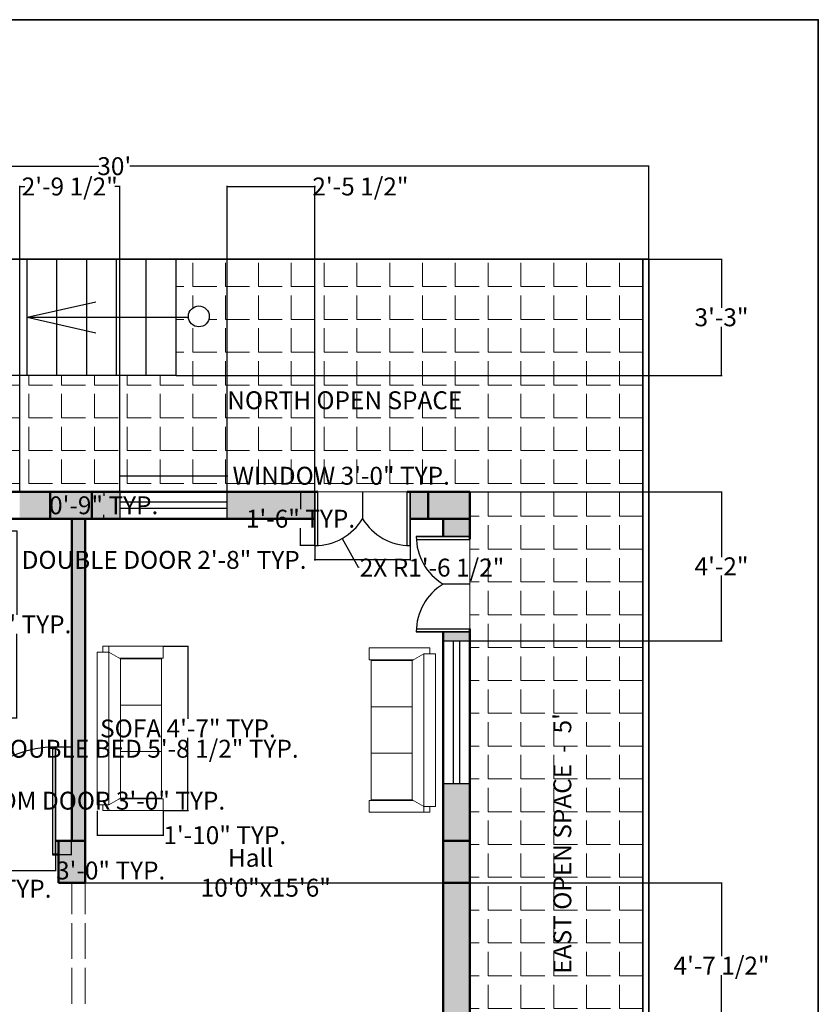
# Model space of a CAD drawing. Units: inches. Extents: x 1601 to 2080, y 5000 to 5589.
# Tile 11 of 11: x 1812 to 2080, y 5259 to 5589. Entities that reach past the tile are written whole.
import ezdxf

# ---------------------------------------------------------------- set-up
doc = ezdxf.new("R2010")
doc.units = ezdxf.units.IN
doc.header["$MEASUREMENT"] = 0
doc.linetypes.add('ACAD_ISO02W100', pattern=[15, 12, -3])
for name, color, linetype, lineweight in [('A-ANNO-DIMS', 2, 'Continuous', 18), ('A-ANNO-TTLB', 7, 'Continuous', 35), ('A-AREA-IDEN', 7, 'Continuous', 25), ('A-COLS', 7, 'Continuous', 50), ('A-COLS-PATT', 18, 'Continuous', 13), ('A-DOOR', 3, 'Continuous', 25), ('A-FLOR-PATT', 8, 'Continuous', 13), ('A-FLOR-STRS', 7, 'Continuous', 25), ('A-FURN', 8, 'Continuous', 18), ('A-GLAZ', 4, 'Continuous', 25), ('A-WALL', 7, 'Continuous', 50), ('A-WALL-OVHD', 7, 'ACAD_ISO02W100', 18), ('A-WALL-PATT', 241, 'Continuous', 13), ('C-PROP', 7, 'Continuous', 35)]:
    doc.layers.add(name, color=color, linetype=linetype, lineweight=lineweight)
doc.styles.get("Standard").update_dxf_attribs({"font": 'arial.ttf'})
doc.dimstyles.get("Standard").update_dxf_attribs({"dimtxt": 6, "dimasz": 0.18, "dimexe": 0.18, "dimexo": 0.0625, "dimgap": 0.09, "dimtad": 0, "dimtih": 1, "dimtoh": 1, "dimdec": 1, "dimzin": 0, "dimdsep": 46, "dimlunit": 3, "dimtxsty": 'Standard', "dimcen": 0.09, "dimadec": 0, "dimazin": 0, "dimtfac": 1, "dimtdec": 1, "dimtofl": 0, "dimtmove": 0, "dimatfit": 3, "dimfxl": 1, "dimtolj": 1, "dimtzin": 0, "dimarcsym": 0})

# ---------------------------------------------------------------- blocks, each defined once
blk = doc.blocks.new('*D3')
at = {"layer": 'A-ANNO-DIMS', "color": 0, "lineweight": -2, "transparency": 16777216}
for p, q in [((1664.41, 5509.26), (1664.41, 5540.54)), ((1664.59, 5540.36), (1838.48, 5540.36)), ((2022.73, 5540.36), (1848.84, 5540.36)), ((2022.91, 5509.26), (2022.91, 5540.54))]:
    blk.add_line(p, q, dxfattribs=at)
at = {"layer": 'A-ANNO-DIMS', "color": 0, "transparency": 16777216}
for points in [[(1664.59, 5540.39), (1664.59, 5540.33), (1664.41, 5540.36)], [(2022.73, 5540.39), (2022.73, 5540.33), (2022.91, 5540.36)]]:
    blk.add_solid(points, dxfattribs=at)
at = {"layer": 'Defpoints', "color": 0, "transparency": 16777216}
for p in [(2022.91, 5540.36), (1664.41, 5509.2), (2022.91, 5509.2)]:
    blk.add_point(p, dxfattribs=at)
at = {"layer": 'A-ANNO-DIMS', "color": 0, "transparency": 16777216, "insert": (1843.66, 5540.36), "char_height": 6, "width": 10.4243, "attachment_point": 5}
blk.add_mtext("\\A1;30'", dxfattribs=at)
blk = doc.blocks.new('SOFA-THREE-SEAT')
for p, q in [((0, 53.08), (0, 1.96)), ((3.92, 53.08), (0, 53.08)), ((1.96, 55.04), (22.23, 55.04)), ((1.96, 55.04), (1.96, 53.08)), ((3.92, 55.04), (3.92, 1.96)), ((3.92, 53.08), (7.85, 50.88)), ((22.23, 51.12), (22.23, 55.04)), ((7.54, 51.12), (22.23, 51.12)), ((21.58, 50.87), (7.85, 50.87)), ((21.58, 35.3), (7.85, 35.3)), ((21.58, 19.74), (7.85, 19.74)), ((7.85, 4.17), (3.92, 1.96)), ((7.29, 3.92), (22.23, 3.92)), ((22.23, 3.92), (22.23, 0)), ((3.92, 1.96), (0, 1.96)), ((1.96, 1.96), (1.96, 0)), ((1.96, 0), (22.23, 0))]:
    blk.add_line(p, q)
blk.add_lwpolyline([(7.85, 50.88), (7.85, 4.17), (21.58, 4.17), (21.58, 50.87)])
blk = doc.blocks.new('DOOR-36IN')
for p, q in [((35, 36), (35, 0)), ((36, 0), (36, 36)), ((36, 36), (36, 0)), ((36, 0), (35, 0))]:
    blk.add_line(p, q)
blk.add_arc((36, -0.32), 36.32, 90, 172.3719)
blk = doc.blocks.new('DOOR-DOUBLE-18IN-LEAVES')
for p, q in [((18, 32), (0, 32)), ((0, 32), (18, 32)), ((0, 31), (18, 31)), ((18, 31), (18, 32)), ((18, 16), (9, 16)), ((0, 1), (18, 1)), ((18, 0), (0, 0)), ((0, 0), (18, 0)), ((18, 0), (18, 1))]:
    blk.add_line(p, q)
for centre, start, end in [((18.72, 32), 180, 238.7155), ((18.72, 0), 121.2845, 180)]:
    blk.add_arc(centre, 18.72, start, end)
blk = doc.blocks.new('WINDOW-48IN')
for p, q in [((0, 0), (0, 9)), ((0, 9), (48, 9)), ((48, 9), (48, 0)), ((0, 5.5), (48, 5.5)), ((48, 3.5), (0, 3.5)), ((48, 0), (0, 0))]:
    blk.add_line(p, q)
blk = doc.blocks.new('WINDOW-36IN')
for p, q in [((0, 9), (0, 0)), ((36, 9), (0, 9)), ((36, 0), (36, 9)), ((36, 5.5), (0, 5.5)), ((0, 3.5), (36, 3.5)), ((0, 0), (36, 0))]:
    blk.add_line(p, q)
blk = doc.blocks.new('*D17')
at = {"layer": 'A-ANNO-DIMS', "color": 0, "lineweight": -2, "transparency": 16777216}
for p, q in [((1731.95, 5355.35), (1731.95, 5344.92)), ((1800.66, 5355.35), (1800.66, 5344.92)), ((1732.13, 5345.1), (1800.48, 5345.1)), ((1800.66, 5345.1), (1800.84, 5345.1))]:
    blk.add_line(p, q, dxfattribs=at)
at = {"layer": 'A-ANNO-DIMS', "color": 0, "transparency": 16777216}
for points in [[(1732.13, 5345.13), (1732.13, 5345.07), (1731.95, 5345.1)], [(1800.48, 5345.13), (1800.48, 5345.07), (1800.66, 5345.1)]]:
    blk.add_solid(points, dxfattribs=at)
at = {"layer": 'Defpoints', "color": 0, "transparency": 16777216}
for p in [(1731.95, 5355.41), (1800.66, 5355.41), (1800.66, 5345.1)]:
    blk.add_point(p, dxfattribs=at)
at = {"layer": 'A-ANNO-DIMS', "color": 0, "transparency": 16777216, "insert": (1854.24, 5345.1), "char_height": 6, "attachment_point": 5}
blk.add_mtext('\\A1;DOUBLE BED 5\'-8 1/2" TYP.', dxfattribs=at)
blk = doc.blocks.new('*D18')
at = {"layer": 'A-ANNO-DIMS', "color": 0, "lineweight": -2, "transparency": 16777216}
for p, q in [((1800.72, 5418.19), (1811.15, 5418.19)), ((1810.97, 5418.01), (1810.97, 5389.96)), ((1810.97, 5355.59), (1810.97, 5383.65)), ((1800.72, 5355.41), (1811.15, 5355.41))]:
    blk.add_line(p, q, dxfattribs=at)
at = {"layer": 'A-ANNO-DIMS', "color": 0, "transparency": 16777216}
for points in [[(1810.94, 5418.01), (1811, 5418.01), (1810.97, 5418.19)], [(1810.94, 5355.59), (1811, 5355.59), (1810.97, 5355.41)]]:
    blk.add_solid(points, dxfattribs=at)
at = {"layer": 'Defpoints', "color": 0, "transparency": 16777216}
for p in [(1800.66, 5418.19), (1810.97, 5418.19), (1800.66, 5355.41)]:
    blk.add_point(p, dxfattribs=at)
at = {"layer": 'A-ANNO-DIMS', "color": 0, "transparency": 16777216, "insert": (1810.97, 5386.8), "char_height": 6, "attachment_point": 5}
blk.add_mtext('\\A1;5\'-3" TYP.', dxfattribs=at)
blk = doc.blocks.new('*D19')
at = {"layer": 'A-ANNO-DIMS', "color": 0, "lineweight": -2, "transparency": 16777216}
for p, q in [((1860.17, 5379.43), (1868.54, 5379.43)), ((1868.36, 5379.25), (1868.36, 5355.1)), ((1868.36, 5324.57), (1868.36, 5348.71)), ((1860.17, 5324.39), (1868.54, 5324.39))]:
    blk.add_line(p, q, dxfattribs=at)
at = {"layer": 'A-ANNO-DIMS', "color": 0, "transparency": 16777216}
for points in [[(1868.33, 5379.25), (1868.39, 5379.25), (1868.36, 5379.43)], [(1868.33, 5324.57), (1868.39, 5324.57), (1868.36, 5324.39)]]:
    blk.add_solid(points, dxfattribs=at)
at = {"layer": 'Defpoints', "color": 0, "transparency": 16777216}
for p in [(1860.11, 5379.43), (1868.36, 5379.43), (1860.11, 5324.39)]:
    blk.add_point(p, dxfattribs=at)
at = {"layer": 'A-ANNO-DIMS', "color": 0, "transparency": 16777216, "insert": (1868.36, 5351.91), "char_height": 6, "attachment_point": 5}
blk.add_mtext('\\A1;SOFA 4\'-7" TYP.', dxfattribs=at)
blk = doc.blocks.new('*D20')
at = {"layer": 'A-ANNO-DIMS', "color": 0, "lineweight": -2, "transparency": 16777216}
for p, q in [((1837.88, 5324.32), (1837.88, 5315.95)), ((1860.11, 5324.32), (1860.11, 5315.95)), ((1838.06, 5316.13), (1859.93, 5316.13)), ((1860.11, 5316.13), (1860.29, 5316.13))]:
    blk.add_line(p, q, dxfattribs=at)
at = {"layer": 'A-ANNO-DIMS', "color": 0, "transparency": 16777216}
for points in [[(1838.06, 5316.16), (1838.06, 5316.1), (1837.88, 5316.13)], [(1859.93, 5316.16), (1859.93, 5316.1), (1860.11, 5316.13)]]:
    blk.add_solid(points, dxfattribs=at)
at = {"layer": 'Defpoints', "color": 0, "transparency": 16777216}
for p in [(1837.88, 5324.39), (1860.11, 5324.39), (1860.11, 5316.13)]:
    blk.add_point(p, dxfattribs=at)
at = {"layer": 'A-ANNO-DIMS', "color": 0, "transparency": 16777216, "insert": (1880.71, 5316.13), "char_height": 6, "attachment_point": 5}
blk.add_mtext('\\A1;1\'-10" TYP.', dxfattribs=at)
blk = doc.blocks.new('*D23')
at = {"layer": 'A-ANNO-DIMS', "color": 0, "lineweight": -2, "transparency": 16777216}
for p, q in [((1823.97, 5345.7), (1829.49, 5345.7)), ((1829.31, 5345.52), (1829.31, 5330.89)), ((1829.31, 5309.88), (1829.31, 5324.5)), ((1823.97, 5309.7), (1829.49, 5309.7))]:
    blk.add_line(p, q, dxfattribs=at)
at = {"layer": 'A-ANNO-DIMS', "color": 0, "transparency": 16777216}
for points in [[(1829.28, 5345.52), (1829.34, 5345.52), (1829.31, 5345.7)], [(1829.28, 5309.88), (1829.34, 5309.88), (1829.31, 5309.7)]]:
    blk.add_solid(points, dxfattribs=at)
at = {"layer": 'Defpoints', "color": 0, "transparency": 16777216}
for p in [(1823.91, 5345.7), (1829.31, 5345.7), (1823.91, 5309.7)]:
    blk.add_point(p, dxfattribs=at)
at = {"layer": 'A-ANNO-DIMS', "color": 0, "transparency": 16777216, "insert": (1829.31, 5327.7), "char_height": 6, "attachment_point": 5}
blk.add_mtext('\\A1;BEDROOM DOOR 3\'-0" TYP.', dxfattribs=at)
blk = doc.blocks.new('*D24')
at = {"layer": 'A-ANNO-DIMS', "color": 0, "lineweight": -2, "transparency": 16777216}
for p, q in [((1787.91, 5309.63), (1787.91, 5304.12)), ((1823.91, 5309.63), (1823.91, 5304.12)), ((1788.09, 5304.3), (1823.73, 5304.3)), ((1823.91, 5304.3), (1824.09, 5304.3))]:
    blk.add_line(p, q, dxfattribs=at)
at = {"layer": 'A-ANNO-DIMS', "color": 0, "transparency": 16777216}
for points in [[(1788.09, 5304.33), (1788.09, 5304.27), (1787.91, 5304.3)], [(1823.73, 5304.33), (1823.73, 5304.27), (1823.91, 5304.3)]]:
    blk.add_solid(points, dxfattribs=at)
at = {"layer": 'Defpoints', "color": 0, "transparency": 16777216}
for p in [(1787.91, 5309.7), (1823.91, 5309.7), (1823.91, 5304.3)]:
    blk.add_point(p, dxfattribs=at)
at = {"layer": 'A-ANNO-DIMS', "color": 0, "transparency": 16777216, "insert": (1842.46, 5304.3), "char_height": 6, "attachment_point": 5}
blk.add_mtext('\\A1;3\'-0" TYP.', dxfattribs=at)
blk = doc.blocks.new('*D25')
at = {"layer": 'A-ANNO-DIMS', "color": 0, "lineweight": -2, "transparency": 16777216}
for p, q in [((1772.47, 5314.2), (1777.39, 5314.2)), ((1777.21, 5314.02), (1777.21, 5301.39)), ((1777.21, 5282.38), (1777.21, 5295)), ((1772.47, 5282.2), (1777.39, 5282.2))]:
    blk.add_line(p, q, dxfattribs=at)
at = {"layer": 'A-ANNO-DIMS', "color": 0, "transparency": 16777216}
for points in [[(1777.18, 5314.02), (1777.24, 5314.02), (1777.21, 5314.2)], [(1777.18, 5282.38), (1777.24, 5282.38), (1777.21, 5282.2)]]:
    blk.add_solid(points, dxfattribs=at)
at = {"layer": 'Defpoints', "color": 0, "transparency": 16777216}
for p in [(1772.41, 5314.2), (1777.21, 5314.2), (1772.41, 5282.2)]:
    blk.add_point(p, dxfattribs=at)
at = {"layer": 'A-ANNO-DIMS', "color": 0, "transparency": 16777216, "insert": (1777.21, 5298.2), "char_height": 6, "attachment_point": 5}
blk.add_mtext('\\A1;TOILET DOOR 2\'-8" TYP.', dxfattribs=at)
blk = doc.blocks.new('*D27')
at = {"layer": 'A-ANNO-DIMS', "color": 0, "lineweight": -2, "transparency": 16777216}
for p, q in [((1910.91, 5413.13), (1910.91, 5408.22)), ((1942.91, 5413.13), (1942.91, 5408.22)), ((1910.91, 5408.4), (1910.73, 5408.4)), ((1942.73, 5408.4), (1911.09, 5408.4))]:
    blk.add_line(p, q, dxfattribs=at)
at = {"layer": 'A-ANNO-DIMS', "color": 0, "transparency": 16777216}
for points in [[(1911.09, 5408.43), (1911.09, 5408.37), (1910.91, 5408.4)], [(1942.73, 5408.43), (1942.73, 5408.37), (1942.91, 5408.4)]]:
    blk.add_solid(points, dxfattribs=at)
at = {"layer": 'Defpoints', "color": 0, "transparency": 16777216}
for p in [(1910.91, 5413.2), (1942.91, 5413.2), (1910.91, 5408.4)]:
    blk.add_point(p, dxfattribs=at)
at = {"layer": 'A-ANNO-DIMS', "color": 0, "transparency": 16777216, "insert": (1860.36, 5408.4), "char_height": 6, "attachment_point": 5}
blk.add_mtext('\\A1;DOUBLE DOOR 2\'-8" TYP.', dxfattribs=at)
blk = doc.blocks.new('*D28')
at = {"layer": 'A-ANNO-DIMS', "color": 0, "lineweight": -2, "transparency": 16777216}
for p, q in [((1910.85, 5431.2), (1905.93, 5431.2)), ((1906.11, 5431.02), (1906.11, 5425.35)), ((1906.11, 5413.38), (1906.11, 5419.04)), ((1910.85, 5413.2), (1905.93, 5413.2))]:
    blk.add_line(p, q, dxfattribs=at)
at = {"layer": 'A-ANNO-DIMS', "color": 0, "transparency": 16777216}
for points in [[(1906.08, 5431.02), (1906.14, 5431.02), (1906.11, 5431.2)], [(1906.08, 5413.38), (1906.14, 5413.38), (1906.11, 5413.2)]]:
    blk.add_solid(points, dxfattribs=at)
at = {"layer": 'Defpoints', "color": 0, "transparency": 16777216}
for p in [(1906.11, 5431.2), (1910.91, 5431.2), (1910.91, 5413.2)]:
    blk.add_point(p, dxfattribs=at)
at = {"layer": 'A-ANNO-DIMS', "color": 0, "transparency": 16777216, "insert": (1906.11, 5422.2), "char_height": 6, "attachment_point": 5}
blk.add_mtext('\\A1;1\'-6" TYP.', dxfattribs=at)
blk = doc.blocks.new('*D29')
at = {"layer": 'A-ANNO-DIMS', "color": 0, "lineweight": -2, "transparency": 16777216}
for p, q in [((1845.52, 5431.26), (1845.52, 5436.78)), ((1845.7, 5436.6), (1881.34, 5436.6)), ((1881.52, 5431.26), (1881.52, 5436.78)), ((1881.52, 5436.6), (1881.7, 5436.6))]:
    blk.add_line(p, q, dxfattribs=at)
at = {"layer": 'A-ANNO-DIMS', "color": 0, "transparency": 16777216}
for points in [[(1845.7, 5436.63), (1845.7, 5436.57), (1845.52, 5436.6)], [(1881.34, 5436.63), (1881.34, 5436.57), (1881.52, 5436.6)]]:
    blk.add_solid(points, dxfattribs=at)
at = {"layer": 'Defpoints', "color": 0, "transparency": 16777216}
for p in [(1881.52, 5436.6), (1845.52, 5431.2), (1881.52, 5431.2)]:
    blk.add_point(p, dxfattribs=at)
at = {"layer": 'A-ANNO-DIMS', "color": 0, "transparency": 16777216, "insert": (1919.76, 5436.6), "char_height": 6, "attachment_point": 5}
blk.add_mtext('\\A1;WINDOW 3\'-0" TYP.', dxfattribs=at)
blk = doc.blocks.new('*D30')
at = {"layer": 'A-ANNO-DIMS', "color": 0, "lineweight": -2, "transparency": 16777216}
for p, q in [((1845.46, 5431.2), (1839.94, 5431.2)), ((1840.12, 5431.02), (1840.12, 5429.85)), ((1845.46, 5422.2), (1839.94, 5422.2)), ((1840.12, 5422.38), (1840.12, 5423.54))]:
    blk.add_line(p, q, dxfattribs=at)
at = {"layer": 'A-ANNO-DIMS', "color": 0, "transparency": 16777216}
for points in [[(1840.09, 5431.02), (1840.15, 5431.02), (1840.12, 5431.2)], [(1840.09, 5422.38), (1840.15, 5422.38), (1840.12, 5422.2)]]:
    blk.add_solid(points, dxfattribs=at)
at = {"layer": 'Defpoints', "color": 0, "transparency": 16777216}
for p in [(1840.12, 5431.2), (1845.52, 5431.2), (1845.52, 5422.2)]:
    blk.add_point(p, dxfattribs=at)
at = {"layer": 'A-ANNO-DIMS', "color": 0, "transparency": 16777216, "insert": (1840.12, 5426.7), "char_height": 6, "attachment_point": 5}
blk.add_mtext('\\A1;0\'-9" TYP.', dxfattribs=at)
blk = doc.blocks.new('*D40')
at = {"layer": 'A-ANNO-DIMS', "color": 0, "lineweight": -2, "transparency": 16777216}
for p, q in [((1864.47, 5509.2), (2047.44, 5509.2)), ((2047.26, 5509.02), (2047.26, 5492.85)), ((2047.26, 5470.38), (2047.26, 5486.54)), ((1864.47, 5470.2), (2047.44, 5470.2))]:
    blk.add_line(p, q, dxfattribs=at)
at = {"layer": 'A-ANNO-DIMS', "color": 0, "transparency": 16777216}
for points in [[(2047.23, 5509.02), (2047.29, 5509.02), (2047.26, 5509.2)], [(2047.23, 5470.38), (2047.29, 5470.38), (2047.26, 5470.2)]]:
    blk.add_solid(points, dxfattribs=at)
at = {"layer": 'Defpoints', "color": 0, "transparency": 16777216}
for p in [(1864.41, 5509.2), (1864.41, 5470.2), (2047.26, 5470.2)]:
    blk.add_point(p, dxfattribs=at)
at = {"layer": 'A-ANNO-DIMS', "color": 0, "transparency": 16777216, "insert": (2047.26, 5489.7), "char_height": 6, "attachment_point": 5}
blk.add_mtext('\\A1;3\'-3"', dxfattribs=at)
blk = doc.blocks.new('*D48')
at = {"layer": 'A-ANNO-DIMS', "color": 0, "lineweight": -2, "transparency": 16777216}
for p, q in [((1811.95, 5431.26), (1811.95, 5533.73)), ((1812.13, 5533.55), (1813.63, 5533.55)), ((1845.34, 5533.55), (1843.84, 5533.55)), ((1845.52, 5431.26), (1845.52, 5533.73))]:
    blk.add_line(p, q, dxfattribs=at)
at = {"layer": 'A-ANNO-DIMS', "color": 0, "transparency": 16777216}
for points in [[(1812.13, 5533.58), (1812.13, 5533.52), (1811.95, 5533.55)], [(1845.34, 5533.58), (1845.34, 5533.52), (1845.52, 5533.55)]]:
    blk.add_solid(points, dxfattribs=at)
at = {"layer": 'Defpoints', "color": 0, "transparency": 16777216}
for p in [(1845.52, 5533.55), (1811.95, 5431.2), (1845.52, 5431.2)]:
    blk.add_point(p, dxfattribs=at)
at = {"layer": 'A-ANNO-DIMS', "color": 0, "transparency": 16777216, "insert": (1828.74, 5533.55), "char_height": 6, "attachment_point": 5}
blk.add_mtext('\\A1;2\'-9 1/2"', dxfattribs=at)
blk = doc.blocks.new('*D49')
at = {"layer": 'A-ANNO-DIMS', "color": 0, "lineweight": -2, "transparency": 16777216}
for p, q in [((1881.52, 5431.26), (1881.52, 5533.73)), ((1881.7, 5533.55), (1910.73, 5533.55)), ((1910.91, 5431.26), (1910.91, 5533.73)), ((1910.91, 5533.55), (1911.09, 5533.55))]:
    blk.add_line(p, q, dxfattribs=at)
at = {"layer": 'A-ANNO-DIMS', "color": 0, "transparency": 16777216}
for points in [[(1881.7, 5533.58), (1881.7, 5533.52), (1881.52, 5533.55)], [(1910.73, 5533.58), (1910.73, 5533.52), (1910.91, 5533.55)]]:
    blk.add_solid(points, dxfattribs=at)
at = {"layer": 'Defpoints', "color": 0, "transparency": 16777216}
for p in [(1910.91, 5533.55), (1881.52, 5431.2), (1910.91, 5431.2)]:
    blk.add_point(p, dxfattribs=at)
at = {"layer": 'A-ANNO-DIMS', "color": 0, "transparency": 16777216, "insert": (1926.19, 5533.55), "char_height": 6, "attachment_point": 5}
blk.add_mtext('\\A1;2\'-5 1/2"', dxfattribs=at)
blk = doc.blocks.new('*D51')
at = {"layer": 'A-ANNO-DIMS', "color": 0, "lineweight": -2, "transparency": 16777216}
for p, q in [((1962.97, 5431.2), (2047.44, 5431.2)), ((2047.26, 5431.02), (2047.26, 5409.34)), ((2047.26, 5381.47), (2047.26, 5403.14)), ((1962.97, 5381.29), (2047.44, 5381.29))]:
    blk.add_line(p, q, dxfattribs=at)
at = {"layer": 'A-ANNO-DIMS', "color": 0, "transparency": 16777216}
for points in [[(2047.23, 5431.02), (2047.29, 5431.02), (2047.26, 5431.2)], [(2047.23, 5381.47), (2047.29, 5381.47), (2047.26, 5381.29)]]:
    blk.add_solid(points, dxfattribs=at)
at = {"layer": 'Defpoints', "color": 0, "transparency": 16777216}
for p in [(1962.91, 5431.2), (2047.26, 5431.2), (1962.91, 5381.29)]:
    blk.add_point(p, dxfattribs=at)
at = {"layer": 'A-ANNO-DIMS', "color": 0, "transparency": 16777216, "insert": (2047.26, 5406.24), "char_height": 6, "attachment_point": 5}
blk.add_mtext('\\A1;4\'-2"', dxfattribs=at)
blk = doc.blocks.new('*D56')
at = {"layer": 'A-ANNO-DIMS', "color": 0, "lineweight": -2, "transparency": 16777216}
for p, q in [((1833.97, 5300.2), (2047.44, 5300.2)), ((2047.26, 5300.02), (2047.26, 5275.61)), ((2047.26, 5244.82), (2047.26, 5269.23)), ((1833.97, 5244.64), (2047.44, 5244.64))]:
    blk.add_line(p, q, dxfattribs=at)
at = {"layer": 'A-ANNO-DIMS', "color": 0, "transparency": 16777216}
for points in [[(2047.23, 5300.02), (2047.29, 5300.02), (2047.26, 5300.2)], [(2047.23, 5244.82), (2047.29, 5244.82), (2047.26, 5244.64)]]:
    blk.add_solid(points, dxfattribs=at)
at = {"layer": 'Defpoints', "color": 0, "transparency": 16777216}
for p in [(1833.91, 5300.2), (2047.26, 5300.2), (1833.91, 5244.64)]:
    blk.add_point(p, dxfattribs=at)
at = {"layer": 'A-ANNO-DIMS', "color": 0, "transparency": 16777216, "insert": (2047.26, 5272.42), "char_height": 6, "attachment_point": 5}
blk.add_mtext('\\A1;4\'-7 1/2"', dxfattribs=at)
blk = doc.blocks.new('*D60')
at = {"layer": 'A-ANNO-DIMS', "color": 0, "lineweight": -2, "transparency": 16777216}
for p, q in [((1785.46, 5353.11), (1785.64, 5353.11)), ((1785.64, 5353.11), (1799.87, 5336.85)), ((1823.82, 5309.37), (1824, 5309.37)), ((1823.91, 5309.28), (1823.91, 5309.46))]:
    blk.add_line(p, q, dxfattribs=at)
at = {"layer": 'A-ANNO-DIMS', "color": 0, "transparency": 16777216}
blk.add_solid([(1799.89, 5336.86), (1799.85, 5336.83), (1799.99, 5336.71)], dxfattribs=at)
at = {"layer": 'Defpoints', "color": 0, "transparency": 16777216}
for p in [(1799.99, 5336.71), (1823.91, 5309.37)]:
    blk.add_point(p, dxfattribs=at)
at = {"layer": 'A-ANNO-DIMS', "color": 0, "transparency": 16777216, "insert": (1767.53, 5353.11), "char_height": 6, "attachment_point": 5}
blk.add_mtext('\\A1;R3\'-0 1/2"', dxfattribs=at)
blk = doc.blocks.new('*D62')
at = {"layer": 'A-ANNO-DIMS', "color": 0, "lineweight": -2, "transparency": 16777216}
for p, q in [((1910.82, 5431.92), (1911, 5431.92)), ((1910.91, 5431.83), (1910.91, 5432.01)), ((1925.59, 5405.81), (1920.18, 5415.44)), ((1925.77, 5405.81), (1925.59, 5405.81))]:
    blk.add_line(p, q, dxfattribs=at)
at = {"layer": 'A-ANNO-DIMS', "color": 0, "transparency": 16777216}
blk.add_solid([(1920.2, 5415.46), (1920.15, 5415.43), (1920.09, 5415.6)], dxfattribs=at)
at = {"layer": 'Defpoints', "color": 0, "transparency": 16777216}
for p in [(1910.91, 5431.92), (1920.09, 5415.6)]:
    blk.add_point(p, dxfattribs=at)
at = {"layer": 'A-ANNO-DIMS', "color": 0, "transparency": 16777216, "insert": (1950.2, 5405.81), "char_height": 6, "attachment_point": 5}
blk.add_mtext('\\A1;2X R1\'-6 1/2"', dxfattribs=at)

msp = doc.modelspace()

# ---------------------------------------------------------------- hatches: boundary and pattern name
at = {"layer": 'A-COLS-PATT'}
h = msp.add_hatch(color=256, dxfattribs=at)
h.dxf.hatch_style = 1
h.paths.add_polyline_path([(1702.41, 5431.2), (1688.41, 5431.2), (1688.41, 5422.2), (1702.41, 5422.2)])
h.paths.add_polyline_path([(1836.17, 5431.2), (1822.17, 5431.2), (1822.17, 5422.2), (1836.17, 5422.2)])
h.paths.add_polyline_path([(1962.91, 5431.2), (1948.91, 5431.2), (1948.91, 5422.2), (1962.91, 5422.2)])
h.paths.add_polyline_path([(1697.41, 5314.2), (1688.41, 5314.2), (1688.41, 5300.2), (1697.41, 5300.2)])
h.paths.add_polyline_path([(1833.91, 5314.2), (1824.91, 5314.2), (1824.91, 5300.2), (1833.91, 5300.2)])
h.paths.add_polyline_path([(1962.91, 5314.2), (1953.91, 5314.2), (1953.91, 5300.2), (1962.91, 5300.2)])
h.paths.add_polyline_path([(1697.41, 5209.2), (1688.41, 5209.2), (1688.41, 5195.2), (1697.41, 5195.2)])
h.paths.add_polyline_path([(1833.91, 5209.2), (1824.91, 5209.2), (1824.91, 5195.2), (1833.91, 5195.2)])
h.paths.add_polyline_path([(1962.91, 5209.2), (1953.91, 5209.2), (1953.91, 5195.2), (1962.91, 5195.2)])
h.paths.add_polyline_path([(1697.41, 5083.7), (1688.41, 5083.7), (1688.41, 5069.7), (1697.41, 5069.7)])
h.paths.add_polyline_path([(1833.91, 5078.7), (1819.91, 5078.7), (1819.91, 5069.7), (1833.91, 5069.7)])
h.paths.add_polyline_path([(1962.91, 5078.7), (1948.91, 5078.7), (1948.91, 5069.7), (1962.91, 5069.7)])
at = {"layer": 'A-FLOR-PATT'}
h = msp.add_hatch(dxfattribs=at)
h.set_pattern_fill('ANGLE', color=256, scale=40)
h.set_pattern_definition([(0, (0, 0), (0, 11), [8, -3]), (90, (0, 0), (-11, 7e-16), [8, -3])])
h.paths.add_polyline_path([(2022.91, 5509.2), (1941.91, 5509.2), (1911.91, 5509.2), (1864.41, 5509.2), (1864.41, 5489.7), (1868.54, 5489.7, -0.022155), (1868.52, 5490.01, -1), (1875.53, 5490.01, -0.956651), (1868.54, 5489.7), (1864.41, 5489.7), (1864.41, 5470.2), (1794.41, 5470.2), (1794.41, 5431.2), (1811.95, 5431.2), (1911.91, 5431.2), (1941.91, 5431.2), (1942.91, 5431.2), (1945.91, 5431.2), (1948.91, 5431.2), (1962.91, 5431.2), (1962.91, 5415.29), (1962.91, 5385.29), (1962.91, 5384.29), (1962.91, 5381.29), (1962.91, 5333.29), (1962.91, 5069.7), (2022.91, 5069.7)])
h.paths.add_polyline_path([(2000.28, 5267.55), (2000.28, 5367.64), (1987.91, 5367.64), (1987.91, 5267.55)], flags=24)
h.paths.add_polyline_path([(1879.42, 5455.52), (1969.04, 5455.52), (1969.04, 5467.88), (1879.42, 5467.88)], flags=24)
at = {"layer": 'A-WALL-PATT'}
h = msp.add_hatch(color=256, dxfattribs=at)
h.dxf.hatch_style = 1
h.paths.add_polyline_path([(1763.95, 5431.2), (1702.41, 5431.2), (1702.41, 5422.2), (1763.95, 5422.2)])
h.paths.add_polyline_path([(1697.41, 5422.2), (1688.41, 5422.2), (1688.41, 5314.2), (1697.41, 5314.2)])
h.paths.add_polyline_path([(1740.41, 5314.2), (1697.41, 5314.2), (1697.41, 5309.7), (1740.41, 5309.7)], flags=17)
h.paths.add_polyline_path([(1822.17, 5431.2), (1811.95, 5431.2), (1811.95, 5422.2), (1822.17, 5422.2)])
h.paths.add_polyline_path([(1845.52, 5431.2), (1836.17, 5431.2), (1836.17, 5422.2), (1845.52, 5422.2)])
h.paths.add_polyline_path([(1910.91, 5431.2), (1881.52, 5431.2), (1881.52, 5422.2), (1910.91, 5422.2)])
h.paths.add_polyline_path([(1948.91, 5431.2), (1945.91, 5431.2), (1942.91, 5431.2), (1942.91, 5422.2), (1948.91, 5422.2)])
h.paths.add_polyline_path([(1962.91, 5422.2), (1953.91, 5422.2), (1953.91, 5416.29), (1962.91, 5416.29)])
h.paths.add_polyline_path([(1962.91, 5384.29), (1953.91, 5384.29), (1953.91, 5381.29), (1962.91, 5381.29)])
h.paths.add_polyline_path([(1962.91, 5333.29), (1953.91, 5333.29), (1953.91, 5314.2), (1962.91, 5314.2)])
h.paths.add_polyline_path([(1962.91, 5300.2), (1953.91, 5300.2), (1953.91, 5236.2), (1875.91, 5236.2), (1875.91, 5230.7), (1881.91, 5230.7), (1881.91, 5231.7), (1953.91, 5231.7), (1953.91, 5219.2), (1962.91, 5219.2)])
h.paths.add_polyline_path([(1962.91, 5185.2), (1953.91, 5185.2), (1953.91, 5183.7), (1881.91, 5183.7), (1881.91, 5184.7), (1875.91, 5184.7), (1875.91, 5183.7), (1875.91, 5179.2), (1953.91, 5179.2), (1953.91, 5172.6), (1962.91, 5172.6)])
h.paths.add_polyline_path([(1962.91, 5136.6), (1953.91, 5136.6), (1953.91, 5078.7), (1962.91, 5078.7)])
h.paths.add_polyline_path([(1948.91, 5078.7), (1833.91, 5078.7), (1833.91, 5069.7), (1948.91, 5069.7)])
h.paths.add_polyline_path([(1833.91, 5195.2), (1829.41, 5195.2), (1829.41, 5078.7), (1833.91, 5078.7)])
h.paths.add_polyline_path([(1819.91, 5078.7), (1813.58, 5078.7), (1813.58, 5069.7), (1819.91, 5069.7)])
h.paths.add_polyline_path([(1765.58, 5078.7), (1697.41, 5078.7), (1697.41, 5069.7), (1765.58, 5069.7)])
h.paths.add_polyline_path([(1697.41, 5195.2), (1688.41, 5195.2), (1688.41, 5083.7), (1697.41, 5083.7)])
h.paths.add_polyline_path([(1740.41, 5209.2), (1697.41, 5209.2), (1697.41, 5204.7), (1740.41, 5204.7)], flags=17)
h.paths.add_polyline_path([(1787.91, 5209.2), (1779.91, 5209.2), (1779.91, 5309.7), (1787.91, 5309.7), (1787.91, 5314.2), (1772.41, 5314.2), (1772.41, 5309.7), (1775.41, 5309.7), (1775.41, 5261.7), (1697.41, 5261.7), (1697.41, 5273.07), (1688.41, 5273.07), (1688.41, 5242.37), (1697.41, 5242.37), (1697.41, 5257.2), (1775.41, 5257.2), (1775.41, 5209.2), (1772.41, 5209.2), (1772.41, 5204.7), (1775.41, 5204.7), (1787.91, 5204.7)])
h.paths.add_polyline_path([(1697.41, 5218.37), (1688.41, 5218.37), (1688.41, 5209.2), (1697.41, 5209.2)], flags=17)
h.paths.add_polyline_path([(1833.91, 5422.2), (1829.41, 5422.2), (1829.41, 5314.2), (1833.91, 5314.2)])
h.paths.add_polyline_path([(1697.41, 5300.2), (1688.41, 5300.2), (1688.41, 5297.07), (1697.41, 5297.07)], flags=17)

# ---------------------------------------------------------------- linework, layer by layer
at = {"layer": 'A-ANNO-TTLB'}
msp.add_lwpolyline([(1600.55, 5589.45), (2079.72, 5589.45), (2079.72, 4999.95), (1600.55, 4999.95)], close=True, dxfattribs=at)
at = {"layer": 'A-COLS'}
for p, q in [((1822.17, 5422.2), (1822.17, 5431.2)), ((1836.17, 5431.2), (1836.17, 5422.2)), ((1948.91, 5431.2), (1948.91, 5422.2)), ((1833.91, 5314.2), (1824.91, 5314.2)), ((1824.91, 5314.2), (1824.91, 5300.2)), ((1953.91, 5314.2), (1962.91, 5314.2)), ((1953.91, 5314.2), (1953.91, 5300.2)), ((1824.91, 5300.2), (1833.91, 5300.2)), ((1953.91, 5300.2), (1962.91, 5300.2))]:
    msp.add_line(p, q, dxfattribs=at)
at = {"layer": 'A-DOOR'}
msp.add_line((1911.91, 5431.2), (1910.91, 5431.2), dxfattribs=at)
at = {"layer": 'A-FLOR-PATT'}
for p, q in [((1911.91, 5431.2), (1941.91, 5431.2)), ((1962.91, 5415.29), (1962.91, 5385.29))]:
    msp.add_line(p, q, dxfattribs=at)
at = {"layer": 'A-FLOR-STRS'}
for p, q in [((1814.41, 5470.2), (1814.41, 5509.2)), ((1824.41, 5470.2), (1824.41, 5509.2)), ((1834.41, 5470.2), (1834.41, 5509.2)), ((1844.41, 5470.2), (1844.41, 5509.2)), ((1854.41, 5470.2), (1854.41, 5509.2)), ((1864.41, 5470.2), (1864.41, 5509.2)), ((1814.41, 5489.7), (1837.5, 5494.87)), ((1814.41, 5489.7), (1868.54, 5489.7)), ((1814.41, 5489.7), (1837.5, 5484.52)), ((1864.41, 5470.2), (1724.41, 5470.2))]:
    msp.add_line(p, q, dxfattribs=at)
msp.add_circle((1872.03, 5490.01), 3.5, dxfattribs=at)
at = {"layer": 'A-WALL'}
for p, q in [((1688.41, 5431.2), (1911.91, 5431.2)), ((1941.91, 5431.2), (1962.91, 5431.2)), ((1945.91, 5431.2), (1942.91, 5431.2)), ((1948.91, 5431.2), (1945.91, 5431.2)), ((1962.91, 5431.2), (1962.91, 5415.29)), ((1688.41, 5422.2), (1910.91, 5422.2)), ((1829.41, 5422.2), (1829.41, 5314.2)), ((1833.91, 5422.2), (1833.91, 5300.2)), ((1942.91, 5422.2), (1962.91, 5422.2)), ((1953.91, 5422.2), (1953.91, 5416.29)), ((1953.91, 5384.29), (1953.91, 5236.2)), ((1962.91, 5385.29), (1962.91, 5069.7)), ((1962.91, 5381.29), (1962.91, 5384.29)), ((1823.91, 5314.2), (1833.91, 5314.2)), ((1822.91, 5309.7), (1824.91, 5309.7)), ((1824.91, 5309.7), (1823.91, 5309.7))]:
    msp.add_line(p, q, dxfattribs=at)
at = {"layer": 'A-WALL-OVHD'}
for p, q in [((1829.41, 5244.64), (1829.41, 5300.2)), ((1833.91, 5244.64), (1833.91, 5300.2))]:
    msp.add_line(p, q, dxfattribs=at)
at = {"layer": 'C-PROP'}
for p, q in [((1664.41, 5509.2), (1911.91, 5509.2)), ((1941.91, 5509.2), (1911.91, 5509.2)), ((1941.91, 5509.2), (2022.91, 5509.2)), ((2020.91, 5509.2), (2020.91, 5047.21)), ((2022.91, 5509.2), (2022.91, 5047.21))]:
    msp.add_line(p, q, dxfattribs=at)

# ---------------------------------------------------------------- block references
at = {"layer": 'A-DOOR', "rotation": 89.99999999999562}
msp.add_blockref('DOOR-DOUBLE-18IN-LEAVES', (1942.91, 5413.2), dxfattribs=at)
at = {"layer": 'A-DOOR'}
for name, p in [('DOOR-DOUBLE-18IN-LEAVES', (1944.91, 5384.28)), ('DOOR-36IN', (1787.91, 5309.7))]:
    msp.add_blockref(name, p, dxfattribs=at)
at = {"layer": 'A-FURN'}
msp.add_blockref('SOFA-THREE-SEAT', (1837.88, 5324.39), dxfattribs=at)
at = {"layer": 'A-FURN', "rotation": 180}
msp.add_blockref('SOFA-THREE-SEAT', (1951.38, 5378.87), dxfattribs=at)
at = {"layer": 'A-GLAZ'}
msp.add_blockref('WINDOW-36IN', (1845.52, 5422.2), dxfattribs=at)
at = {"layer": 'A-GLAZ', "rotation": 269.9999999999983}
msp.add_blockref('WINDOW-48IN', (1953.91, 5381.29), dxfattribs=at)

# ---------------------------------------------------------------- texts
at = {"layer": 'A-AREA-IDEN', "char_height": 6, "attachment_point": 1}
for s, width, insert in [('\\pxt10;NORTH OPEN SPACE', 93.8151, (1881.56, 5464.9)), ('     Hall\\P10\'0"x15\'6"', 44.2051, (1872.63, 5311.53))]:
    msp.add_mtext_dynamic_manual_height_columns(s, width=width, gutter_width=30, heights=[0], dxfattribs=dict(at, insert=insert))
at = {"layer": 'A-AREA-IDEN', "insert": (1990.89, 5269.72), "char_height": 6, "attachment_point": 1, "rotation": 90}
msp.add_mtext_dynamic_manual_height_columns("EAST OPEN SPACE  -  5'", width=171.349, gutter_width=30, heights=[0], dxfattribs=at)

# ---------------------------------------------------------------- dimensions: what is measured, and where the dimension line sits
at = {"layer": 'A-ANNO-DIMS'}
for base, p1, p2, text, override, picture, middle in [((2022.91, 5540.36), (1664.41, 5509.2), (2022.91, 5509.2), "30'", {"dimclrd": 0, "dimclre": 0, "dimclrt": 0}, '*D3', (1843.66, 5540.36)), ((1881.52, 5436.6), (1845.52, 5431.2), (1881.52, 5431.2), 'WINDOW <> TYP.', {"dimdec": 1, "dimlfac": 1, "dimrnd": 0, "dimzin": 1, "dimdsep": 46, "dimlunit": 4, "dimfrac": 2}, '*D29', (1919.76, 5436.6)), ((1800.66, 5345.1), (1731.95, 5355.41), (1800.66, 5355.41), 'DOUBLE BED <> TYP.', {"dimdec": 1, "dimlfac": 1, "dimrnd": 0, "dimzin": 1, "dimdsep": 46, "dimlunit": 4, "dimfrac": 2}, '*D17', (1854.24, 5345.1)), ((1860.11, 5316.13), (1837.88, 5324.39), (1860.11, 5324.39), '<> TYP.', {"dimdec": 1, "dimlfac": 1, "dimrnd": 0, "dimzin": 1, "dimdsep": 46, "dimlunit": 4, "dimfrac": 2}, '*D20', (1880.71, 5316.13)), ((1823.91, 5304.3), (1787.91, 5309.7), (1823.91, 5309.7), '<> TYP.', {"dimdec": 1, "dimlfac": 1, "dimrnd": 0, "dimzin": 1, "dimdsep": 46, "dimlunit": 4, "dimfrac": 2}, '*D24', (1842.46, 5304.3))]:
    dim = msp.add_linear_dim(base=base, p1=p1, p2=p2, text=text, dimstyle='Standard', override=override, dxfattribs=at)
    dim.commit()
    dim.dimension.update_dxf_attribs({"geometry": picture, "text_midpoint": middle})
for base, p1, p2, picture, middle in [((1845.52, 5533.55), (1811.95, 5431.2), (1845.52, 5431.2), '*D48', (1828.74, 5533.55)), ((1910.91, 5533.55), (1881.52, 5431.2), (1910.91, 5431.2), '*D49', (1926.19, 5533.55))]:
    dim = msp.add_linear_dim(base=base, p1=p1, p2=p2, dimstyle='Standard', override={"dimdec": 1, "dimlfac": 1, "dimrnd": 0, "dimzin": 1, "dimdsep": 46, "dimlunit": 4, "dimfrac": 2}, dxfattribs=at)
    dim.commit()
    dim.dimension.update_dxf_attribs({"geometry": picture, "text_midpoint": middle})
for base, p1, p2, picture, middle in [((2047.26, 5470.2), (1864.41, 5509.2), (1864.41, 5470.2), '*D40', (2047.26, 5489.7)), ((2047.26, 5431.2), (1962.91, 5381.29), (1962.91, 5431.2), '*D51', (2047.26, 5406.24)), ((2047.26, 5300.2), (1833.91, 5244.64), (1833.91, 5300.2), '*D56', (2047.26, 5272.42))]:
    dim = msp.add_linear_dim(base=base, p1=p1, p2=p2, angle=90, dimstyle='Standard', override={"dimdec": 1, "dimlfac": 1, "dimrnd": 0, "dimzin": 1, "dimdsep": 46, "dimlunit": 4, "dimfrac": 2}, dxfattribs=at)
    dim.commit()
    dim.dimension.update_dxf_attribs({"geometry": picture, "text_midpoint": middle})
for base, p1, p2, angle, text, picture, middle in [((1840.12, 5431.2), (1845.52, 5422.2), (1845.52, 5431.2), 90, '<> TYP.', '*D30', (1840.12, 5426.7)), ((1906.11, 5431.2), (1910.91, 5413.2), (1910.91, 5431.2), 90, '<> TYP.', '*D28', (1906.11, 5422.2)), ((1910.91, 5408.4), (1942.91, 5413.2), (1910.91, 5413.2), 180, 'DOUBLE DOOR <> TYP.', '*D27', (1860.36, 5408.4)), ((1810.97, 5418.19), (1800.66, 5355.41), (1800.66, 5418.19), 90, '<> TYP.', '*D18', (1810.97, 5386.8)), ((1868.36, 5379.43), (1860.11, 5324.39), (1860.11, 5379.43), 90, 'SOFA <> TYP.', '*D19', (1868.36, 5351.91)), ((1829.31, 5345.7), (1823.91, 5309.7), (1823.91, 5345.7), 90, 'BEDROOM DOOR <> TYP.', '*D23', (1829.31, 5327.7)), ((1777.21, 5314.2), (1772.41, 5282.2), (1772.41, 5314.2), 90, 'TOILET DOOR <> TYP.', '*D25', (1777.21, 5298.2))]:
    dim = msp.add_linear_dim(base=base, p1=p1, p2=p2, angle=angle, text=text, dimstyle='Standard', override={"dimdec": 1, "dimlfac": 1, "dimrnd": 0, "dimzin": 1, "dimdsep": 46, "dimlunit": 4, "dimfrac": 2}, dxfattribs=at)
    dim.commit()
    dim.dimension.update_dxf_attribs({"geometry": picture, "text_midpoint": middle})
dim = msp.add_radius_dim(center=(1910.91, 5431.92), mpoint=(1920.09, 5415.6), text='2X <>', dimstyle='Standard', override={"dimdec": 1, "dimlfac": 1, "dimrnd": 0, "dimzin": 1, "dimdsep": 46, "dimlunit": 4, "dimfrac": 2}, dxfattribs=at)
dim.commit()
dim.dimension.update_dxf_attribs({"geometry": '*D62', "text_midpoint": (1950.2, 5405.81), "dimtype": 164})
dim = msp.add_radius_dim(center=(1823.91, 5309.37), mpoint=(1799.99, 5336.71), dimstyle='Standard', override={"dimdec": 1, "dimlfac": 1, "dimrnd": 0, "dimzin": 1, "dimdsep": 46, "dimlunit": 4, "dimfrac": 2}, dxfattribs=at)
dim.commit()
dim.dimension.update_dxf_attribs({"geometry": '*D60', "text_midpoint": (1767.53, 5353.11), "dimtype": 164})

doc.saveas('drawing.dxf')
